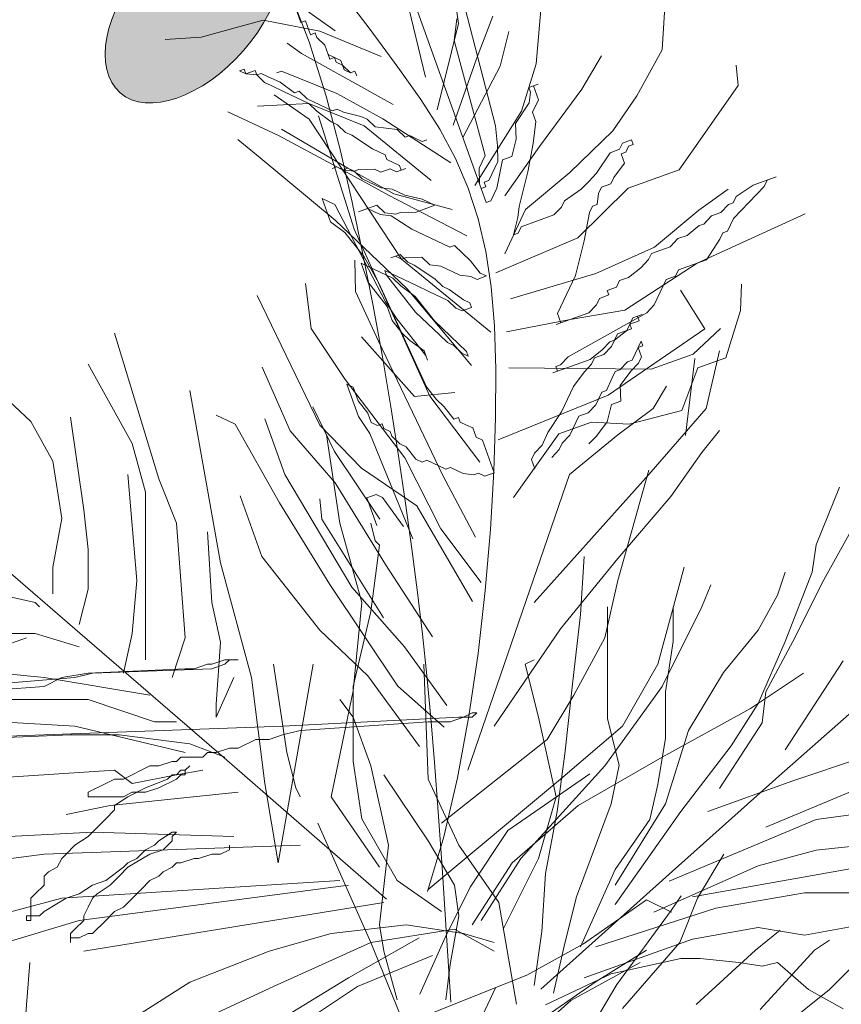
# Model space of a CAD drawing. Units: millimetres. Extents: x 595116 to 630915, y 909473 to 920225.
# Tile 101 of 134: x 629803.095 to 629807.854, y 919172.019 to 919177.721. Entities that reach past the tile are written whole.
import ezdxf

# ---------------------------------------------------------------- set-up
doc = ezdxf.new("R2010")
doc.units = ezdxf.units.MM
doc.layers.add('L-PLNT', color=85, linetype='Continuous', lineweight=13)

# ---------------------------------------------------------------- blocks, each defined once
blk = doc.blocks.new('A$C4FB75ABC')
for p, q in [((2.7169, 3.7399), (2.6018, 4.2172)), ((2.8029, 3.5683), (2.5783, 4.1926)), ((2.7679, 3.8231), (2.7507, 3.9385)), ((2.7636, 3.9026), (2.8247, 3.6653)), ((2.5777, 3.8114), (2.4796, 3.8815)), ((2.5372, 3.7949), (2.5035, 3.8821)), ((2.5794, 3.8826), (2.6314, 3.8136)), ((2.8876, 3.7608), (2.897, 3.8696)), ((2.5166, 3.8462), (2.5244, 3.8247)), ((2.4664, 3.8281), (2.3706, 3.8017)), ((2.5536, 3.8109), (2.4664, 3.8281)), ((2.7613, 3.7965), (2.7653, 3.8303)), ((2.7957, 3.7683), (2.8207, 3.834)), ((3.0823, 3.7823), (3.0858, 3.8403)), ((2.5244, 3.8247), (2.5315, 3.8272)), ((2.5315, 3.8272), (2.5393, 3.8057)), ((2.6314, 3.8136), (2.6743, 3.7558)), ((2.7349, 3.6897), (2.7679, 3.8231)), ((2.3706, 3.8017), (2.3152, 3.798)), ((2.5393, 3.8057), (2.5464, 3.8083)), ((2.5464, 3.8083), (2.549, 3.8011)), ((2.549, 3.8011), (2.5614, 3.7893)), ((2.6486, 3.7721), (2.5536, 3.8109)), ((2.8322, 3.7571), (2.8454, 3.8105)), ((2.5255, 3.7764), (2.5034, 3.7928)), ((2.5638, 3.7106), (2.5372, 3.7949)), ((2.5614, 3.7893), (2.5665, 3.775)), ((2.8089, 3.6191), (2.7613, 3.7965)), ((2.6672, 3.6978), (2.5255, 3.7764)), ((2.5665, 3.775), (2.5763, 3.7704)), ((2.5691, 3.7678), (2.5665, 3.775)), ((2.5763, 3.7704), (2.5691, 3.7678)), ((2.5763, 3.7704), (2.5789, 3.7632)), ((2.586, 3.7658), (2.5763, 3.7704)), ((2.7596, 3.6662), (2.7957, 3.7683)), ((2.9584, 3.7215), (2.9885, 3.7729)), ((3.043, 3.7114), (3.0823, 3.7823)), ((2.4369, 3.7526), (2.4297, 3.7501)), ((2.4394, 3.7455), (2.4369, 3.7526)), ((2.5789, 3.7632), (2.5886, 3.7586)), ((2.5886, 3.7586), (2.586, 3.7658)), ((2.5886, 3.7586), (2.5912, 3.7515)), ((2.601, 3.7469), (2.5886, 3.7586)), ((2.6743, 3.7558), (2.7096, 3.7056)), ((2.7745, 3.6472), (2.8322, 3.7571)), ((2.8652, 3.6879), (2.8876, 3.7608)), ((3.1994, 3.7272), (3.1962, 3.7584)), ((2.4297, 3.7501), (2.4394, 3.7455)), ((2.4538, 3.7506), (2.4394, 3.7455)), ((2.4394, 3.7455), (2.4564, 3.7435)), ((2.4564, 3.7435), (2.4538, 3.7506)), ((2.4635, 3.746), (2.4564, 3.7435)), ((2.4564, 3.7435), (2.4687, 3.7317)), ((2.4733, 3.7414), (2.4635, 3.746)), ((2.4928, 3.7323), (2.4733, 3.7414)), ((2.4948, 3.7492), (2.4876, 3.7466)), ((2.58, 3.715), (2.4948, 3.7492)), ((2.5912, 3.7515), (2.601, 3.7469)), ((2.601, 3.7469), (2.6081, 3.7494)), ((2.6081, 3.7494), (2.601, 3.7469)), ((2.6081, 3.7494), (2.6107, 3.7423)), ((2.6107, 3.7423), (2.6081, 3.7494)), ((2.4687, 3.7317), (2.4785, 3.7271)), ((2.4785, 3.7271), (2.498, 3.7179)), ((2.5149, 3.7159), (2.4928, 3.7323)), ((2.8907, 3.7295), (2.8764, 3.7244)), ((2.8764, 3.7244), (2.8789, 3.7172)), ((2.8835, 3.727), (2.8907, 3.7295)), ((2.8913, 3.7054), (2.8835, 3.727)), ((3.1085, 3.5972), (3.1994, 3.7272)), ((2.5376, 3.6754), (2.4836, 3.7127)), ((2.498, 3.7179), (2.5272, 3.7041)), ((2.5221, 3.7185), (2.5149, 3.7159)), ((2.5344, 3.7067), (2.5221, 3.7185)), ((2.5441, 3.7021), (2.5344, 3.7067)), ((2.5853, 3.6284), (2.5638, 3.7106)), ((2.6509, 3.6757), (2.58, 3.715)), ((2.8789, 3.7172), (2.8769, 3.7003)), ((2.893, 3.6331), (2.9584, 3.7215)), ((3.0058, 3.6575), (3.043, 3.7114)), ((2.537, 3.6995), (2.4575, 3.6952)), ((2.5272, 3.7041), (2.537, 3.6995)), ((2.537, 3.6995), (2.5493, 3.6877)), ((2.6222, 3.6653), (2.537, 3.6995)), ((2.5637, 3.6929), (2.5441, 3.7021)), ((2.5734, 3.6883), (2.5637, 3.6929)), ((2.7096, 3.7056), (2.7388, 3.6597)), ((2.8769, 3.7003), (2.856, 3.6684)), ((2.8821, 3.6859), (2.8913, 3.7054)), ((2.4899, 3.6502), (2.4119, 3.6869)), ((2.5493, 3.6877), (2.5714, 3.6714)), ((2.6067, 3.5058), (2.5519, 3.6806)), ((2.5806, 3.6909), (2.5734, 3.6883)), ((2.5903, 3.6863), (2.5806, 3.6909)), ((2.617, 3.6797), (2.5903, 3.6863)), ((2.6268, 3.6751), (2.617, 3.6797)), ((2.7932, 3.5729), (2.8652, 3.6879)), ((2.8873, 3.6716), (2.8821, 3.6859)), ((2.6801, 3.4593), (2.5376, 3.6754)), ((2.5714, 3.6714), (2.5812, 3.6668)), ((2.5812, 3.6668), (2.5935, 3.655)), ((2.7255, 3.5809), (2.6222, 3.6653)), ((2.6391, 3.6633), (2.6268, 3.6751)), ((2.673, 3.6593), (2.6391, 3.6633)), ((2.7562, 3.6082), (2.6509, 3.6757)), ((2.8247, 3.6653), (2.8279, 3.634)), ((2.856, 3.6684), (2.8566, 3.6443)), ((2.8833, 3.6377), (2.8873, 3.6716)), ((2.5803, 3.6016), (2.4899, 3.6502)), ((2.5972, 3.5996), (2.4945, 3.6599)), ((2.5935, 3.655), (2.6032, 3.6504)), ((2.6032, 3.6504), (2.6351, 3.6295)), ((2.6853, 3.6475), (2.673, 3.6593)), ((2.6925, 3.6501), (2.6853, 3.6475)), ((2.7022, 3.6455), (2.6925, 3.6501)), ((2.7388, 3.6597), (2.763, 3.6147)), ((2.9398, 3.5932), (3.0058, 3.6575)), ((2.4618, 3.6157), (2.4274, 3.6439)), ((2.712, 3.6409), (2.7022, 3.6455)), ((2.7192, 3.6435), (2.712, 3.6409)), ((2.8279, 3.634), (2.8285, 3.6099)), ((2.8394, 3.5571), (2.893, 3.6331)), ((2.8566, 3.6443), (2.85, 3.6176)), ((2.8746, 3.5941), (2.8833, 3.6377)), ((3.0207, 3.6385), (3.0161, 3.6288)), ((3.035, 3.6437), (3.0207, 3.6385)), ((3.0258, 3.6242), (3.0304, 3.6339)), ((3.0304, 3.6339), (3.0376, 3.6365)), ((3.0376, 3.6365), (3.035, 3.6437)), ((2.5774, 3.5196), (2.4618, 3.6157)), ((2.6037, 3.5475), (2.5853, 3.6284)), ((2.6351, 3.6295), (2.6448, 3.6249)), ((2.6448, 3.6249), (2.6546, 3.6203)), ((2.6546, 3.6203), (2.6572, 3.6131)), ((2.7998, 3.5996), (2.8089, 3.6191)), ((2.85, 3.6176), (2.8356, 3.6125)), ((3.0017, 3.6236), (2.9808, 3.5918)), ((3.0161, 3.6288), (3.0017, 3.6236)), ((3.0187, 3.6216), (3.0258, 3.6242)), ((3.0238, 3.6072), (3.0187, 3.6216)), ((2.5803, 3.6016), (2.5731, 3.5991)), ((2.5731, 3.5991), (2.5803, 3.6016)), ((2.5901, 3.597), (2.5803, 3.6016)), ((2.5803, 3.6016), (2.5901, 3.597)), ((2.6609, 3.5577), (2.5803, 3.6016)), ((2.6572, 3.6131), (2.6669, 3.6085)), ((2.6669, 3.6085), (2.6767, 3.6039)), ((2.6767, 3.6039), (2.6793, 3.5967)), ((2.763, 3.6147), (2.7827, 3.5691)), ((2.8285, 3.6099), (2.8193, 3.5904)), ((2.8356, 3.6125), (2.827, 3.5688)), ((3.0075, 3.5852), (3.0238, 3.6072)), ((2.5972, 3.5996), (2.5901, 3.597)), ((2.5901, 3.597), (2.607, 3.595)), ((2.607, 3.595), (2.5972, 3.5996)), ((2.6681, 3.5603), (2.5972, 3.5996)), ((2.6142, 3.5976), (2.607, 3.595)), ((2.607, 3.595), (2.6193, 3.5833)), ((2.6383, 3.5982), (2.6142, 3.5976)), ((2.648, 3.5936), (2.6383, 3.5982)), ((2.6623, 3.5987), (2.648, 3.5936)), ((2.6721, 3.5942), (2.6623, 3.5987)), ((2.6864, 3.5993), (2.6721, 3.5942)), ((2.6793, 3.5967), (2.6864, 3.5993)), ((2.8003, 3.5755), (2.7998, 3.5996)), ((2.8193, 3.5904), (2.8147, 3.5806)), ((2.868, 3.5674), (2.8746, 3.5941)), ((2.8712, 3.5361), (2.9398, 3.5932)), ((2.9808, 3.5918), (2.969, 3.5794)), ((3.0029, 3.5754), (3.0075, 3.5852)), ((3.0296, 3.5688), (3.1085, 3.5972)), ((3.2582, 3.5862), (3.2224, 3.5733)), ((3.2439, 3.5811), (3.2582, 3.5862)), ((2.6193, 3.5833), (2.6486, 3.5695)), ((2.8107, 3.5468), (2.8003, 3.5755)), ((2.8101, 3.5709), (2.8029, 3.5683)), ((2.8147, 3.5806), (2.8075, 3.578)), ((2.8075, 3.578), (2.8101, 3.5709)), ((2.969, 3.5794), (2.9573, 3.5671)), ((2.984, 3.5605), (2.9885, 3.5702)), ((2.9885, 3.5702), (3.0029, 3.5754)), ((3.2224, 3.5733), (3.1962, 3.5558)), ((3.2158, 3.5466), (3.2393, 3.5713)), ((3.2393, 3.5713), (3.2439, 3.5811)), ((2.6486, 3.5695), (2.6655, 3.5675)), ((2.7805, 3.4954), (2.6609, 3.5577)), ((2.6655, 3.5675), (2.685, 3.5583)), ((2.7579, 3.5359), (2.6681, 3.5603)), ((2.685, 3.5583), (2.7117, 3.5517)), ((2.7827, 3.5691), (2.7983, 3.5216)), ((2.8224, 3.5591), (2.8178, 3.5493)), ((2.827, 3.5688), (2.8224, 3.5591)), ((2.8614, 3.5407), (2.868, 3.5674)), ((2.9573, 3.5671), (2.9312, 3.5496)), ((2.9518, 3.4922), (3.0296, 3.5688)), ((2.9819, 3.5435), (2.984, 3.5605)), ((3.1389, 3.5352), (3.1839, 3.5676)), ((3.1962, 3.5558), (3.1917, 3.5461)), ((2.5671, 3.5483), (2.5573, 3.5529)), ((2.5573, 3.5529), (2.5703, 3.517)), ((2.5769, 3.5437), (2.5671, 3.5483)), ((2.6552, 3.3935), (2.5769, 3.5437)), ((2.6204, 3.467), (2.6037, 3.5475)), ((2.642, 3.5428), (2.6133, 3.5325)), ((2.6543, 3.531), (2.642, 3.5428)), ((2.7312, 3.5425), (2.7025, 3.5321)), ((2.7117, 3.5517), (2.7214, 3.5471)), ((2.7214, 3.5471), (2.7312, 3.5425)), ((2.8178, 3.5493), (2.8107, 3.5468)), ((2.8594, 3.5238), (2.8614, 3.5407)), ((2.9266, 3.5398), (2.9148, 3.5275)), ((2.9312, 3.5496), (2.9266, 3.5398)), ((2.9702, 3.5312), (2.9748, 3.541)), ((2.9748, 3.541), (2.9819, 3.5435)), ((3.1845, 3.5435), (3.1727, 3.5311)), ((3.1917, 3.5461), (3.1845, 3.5435)), ((3.1922, 3.522), (3.2158, 3.5466)), ((2.6133, 3.5325), (2.6276, 3.5376)), ((2.6276, 3.5376), (2.6471, 3.5284)), ((2.6471, 3.5284), (2.6641, 3.5264)), ((2.6712, 3.529), (2.6543, 3.531)), ((2.6641, 3.5264), (2.6959, 3.5055)), ((2.6784, 3.5316), (2.6712, 3.529)), ((2.7025, 3.5321), (2.6784, 3.5316)), ((2.8391, 3.4678), (2.8712, 3.5361)), ((2.9148, 3.5275), (2.8646, 3.5094)), ((2.9616, 3.4876), (2.9702, 3.5312)), ((3.0703, 3.4781), (3.1389, 3.5352)), ((3.136, 3.4531), (3.303, 3.5294)), ((3.1584, 3.526), (3.1466, 3.5136)), ((3.1727, 3.5311), (3.1584, 3.526)), ((2.5703, 3.517), (2.5924, 3.5006)), ((2.6885, 3.4136), (2.5774, 3.5196)), ((2.7983, 3.5216), (2.81, 3.4712)), ((2.8528, 3.4971), (2.8594, 3.5238)), ((2.8646, 3.5094), (2.86, 3.4997)), ((3.1394, 3.5111), (3.1205, 3.4961)), ((3.1466, 3.5136), (3.1394, 3.5111)), ((3.1831, 3.5024), (3.1922, 3.522)), ((2.5924, 3.5006), (2.6222, 3.4627)), ((2.7237, 3.248), (2.6067, 3.5058)), ((2.6959, 3.5055), (2.7154, 3.4963)), ((2.7154, 3.4963), (2.7252, 3.4917)), ((2.86, 3.4997), (2.8528, 3.4971)), ((3.1205, 3.4961), (3.1062, 3.491)), ((3.1713, 3.4901), (3.1759, 3.4999)), ((3.1759, 3.4999), (3.1831, 3.5024)), ((2.7252, 3.4917), (2.7544, 3.4779)), ((2.7544, 3.4779), (2.7616, 3.4805)), ((2.7616, 3.4805), (2.774, 3.4687)), ((2.8253, 3.4385), (2.9518, 3.4922)), ((2.9484, 3.4342), (2.9616, 3.4876)), ((3.0944, 3.4786), (3.0657, 3.4683)), ((3.1062, 3.491), (3.0944, 3.4786)), ((3.1503, 3.4583), (3.1713, 3.4901)), ((2.636, 3.3873), (2.6204, 3.467)), ((2.6632, 3.4613), (2.6776, 3.4664)), ((2.6704, 3.4639), (2.6632, 3.4613)), ((2.6801, 3.4593), (2.6704, 3.4639)), ((2.6776, 3.4664), (2.6899, 3.4547)), ((2.774, 3.4687), (2.7863, 3.4569)), ((2.81, 3.4712), (2.8183, 3.4166)), ((2.9797, 3.4374), (3.0703, 3.4781)), ((3.0657, 3.4683), (3.0611, 3.4586)), ((2.609, 3.4093), (2.6078, 3.4576)), ((2.6566, 3.4346), (2.6176, 3.453)), ((2.6176, 3.453), (2.6279, 3.4243)), ((2.6222, 3.4627), (2.6449, 3.4222)), ((2.6873, 3.4618), (2.6801, 3.4593)), ((2.8178, 3.3467), (2.6801, 3.4593)), ((2.7114, 3.4624), (2.6873, 3.4618)), ((2.6899, 3.4547), (2.6996, 3.4501)), ((2.6996, 3.4501), (2.7315, 3.4291)), ((2.7237, 3.4506), (2.7114, 3.4624)), ((2.7407, 3.4486), (2.7237, 3.4506)), ((2.7699, 3.4348), (2.7407, 3.4486)), ((2.7863, 3.4569), (2.8012, 3.438)), ((3.0244, 3.3805), (3.136, 3.4531)), ((3.0611, 3.4586), (3.0494, 3.4462)), ((3.1073, 3.4428), (3.1503, 3.4583)), ((2.6638, 3.4372), (2.654, 3.4418)), ((2.654, 3.4418), (2.6566, 3.4346)), ((2.6566, 3.4346), (2.6664, 3.43)), ((2.6865, 3.3967), (2.6566, 3.4346)), ((2.693, 3.4234), (2.6638, 3.4372)), ((2.7869, 3.4328), (2.7699, 3.4348)), ((2.811, 3.4334), (2.7966, 3.4282)), ((2.8012, 3.438), (2.811, 3.4334)), ((2.848, 3.3981), (2.9797, 3.4374)), ((2.9392, 3.4147), (2.9484, 3.4342)), ((3.0494, 3.4462), (3.0304, 3.4313)), ((3.1027, 3.433), (3.1073, 3.4428)), ((2.5404, 3.3522), (2.5315, 3.422)), ((2.6279, 3.4243), (2.6578, 3.3864)), ((2.6449, 3.4222), (2.7186, 3.2624)), ((2.6664, 3.43), (2.6787, 3.4182)), ((2.6787, 3.4182), (2.7008, 3.4019)), ((2.7028, 3.4188), (2.693, 3.4234)), ((2.7223, 3.4096), (2.7028, 3.4188)), ((2.7315, 3.4291), (2.7438, 3.4173)), ((2.7966, 3.4282), (2.7869, 3.4328)), ((3.0161, 3.4262), (3.0115, 3.4164)), ((3.0304, 3.4313), (3.0161, 3.4262)), ((3.07, 3.3888), (3.0884, 3.4279)), ((3.0884, 3.4279), (3.1027, 3.433)), ((3.2028, 3.3799), (3.2043, 3.4209)), ((2.5536, 3.203), (2.4572, 3.4034)), ((2.6446, 3.333), (2.609, 3.4093)), ((2.7877, 3.2953), (2.6885, 3.4136)), ((2.7516, 3.3958), (2.7223, 3.4096)), ((2.7438, 3.4173), (2.7536, 3.4127)), ((2.7536, 3.4127), (2.7757, 3.3964)), ((2.8183, 3.4166), (2.8233, 3.3565)), ((2.9254, 3.3854), (2.9392, 3.4147)), ((2.9997, 3.4041), (2.9854, 3.3989)), ((3.0115, 3.4164), (2.9972, 3.4112)), ((2.9972, 3.4112), (2.9997, 3.4041)), ((3.1481, 3.3521), (3.1105, 3.4115)), ((2.6727, 3.3674), (2.6552, 3.3935)), ((2.7014, 3.3777), (2.6865, 3.3967)), ((2.7008, 3.4019), (2.7306, 3.364)), ((2.7639, 3.384), (2.7516, 3.3958)), ((2.7757, 3.3964), (2.7854, 3.3918)), ((2.7854, 3.3918), (2.788, 3.3846)), ((2.9808, 3.3891), (2.969, 3.3768)), ((2.9854, 3.3989), (2.9808, 3.3891)), ((3.0583, 3.3765), (3.07, 3.3888)), ((2.6503, 3.3086), (2.636, 3.3873)), ((2.6578, 3.3864), (2.6655, 3.3648)), ((2.7384, 3.3424), (2.7014, 3.3777)), ((2.7737, 3.3794), (2.7639, 3.384)), ((2.788, 3.3846), (2.7737, 3.3794)), ((2.969, 3.3768), (2.9188, 3.3587)), ((2.9208, 3.3757), (2.9254, 3.3854)), ((2.926, 3.3613), (2.9208, 3.3757)), ((2.9369, 3.3085), (3.0583, 3.3765)), ((2.9403, 3.3665), (3.0244, 3.3805)), ((3.0511, 3.3739), (3.0367, 3.3687)), ((3.0439, 3.3713), (3.0511, 3.3739)), ((3.1805, 3.307), (3.2028, 3.3799)), ((2.6655, 3.3648), (2.6804, 3.3459)), ((2.7174, 3.3106), (2.6727, 3.3674)), ((2.7306, 3.364), (2.743, 3.3522)), ((2.8419, 3.3473), (2.9403, 3.3665)), ((2.9188, 3.3587), (2.926, 3.3613)), ((3.0322, 3.359), (3.0276, 3.3492)), ((3.0367, 3.3687), (3.0322, 3.359)), ((3.0322, 3.359), (3.0465, 3.3642)), ((3.0347, 3.3518), (3.0322, 3.359)), ((3.0465, 3.3642), (3.0439, 3.3713)), ((2.2372, 3.345), (2.3054, 3.1203)), ((2.5929, 3.2739), (2.5404, 3.3522)), ((2.6804, 3.3459), (2.6928, 3.3341)), ((2.7507, 3.3307), (2.7384, 3.3424)), ((2.743, 3.3522), (2.7553, 3.3404)), ((2.8233, 3.3565), (2.8254, 3.2898)), ((2.9986, 3.2497), (3.1481, 3.3521)), ((3.0276, 3.3492), (3.0086, 3.3343)), ((3.0086, 3.3343), (3.0132, 3.3441)), ((3.0132, 3.3441), (3.0347, 3.3518)), ((3.1297, 3.313), (3.1722, 3.3526)), ((2.6997, 3.2474), (2.6179, 3.3396)), ((2.7435, 3.1255), (2.6446, 3.333)), ((2.6928, 3.3341), (2.7149, 3.3178)), ((2.7605, 3.3261), (2.7507, 3.3307)), ((2.7553, 3.3404), (2.78, 3.3169)), ((3.0015, 3.3317), (2.9897, 3.3194)), ((3.0086, 3.3343), (3.0015, 3.3317)), ((3.004, 3.3246), (3.0086, 3.3343)), ((3.0497, 3.3329), (3.0451, 3.3231)), ((3.0522, 3.3257), (3.0497, 3.3329)), ((2.7149, 3.3178), (2.72, 3.3034)), ((2.7728, 3.3143), (2.7605, 3.3261)), ((2.7826, 3.3097), (2.7728, 3.3143)), ((2.78, 3.3169), (2.7826, 3.3097)), ((2.9897, 3.3194), (2.9708, 3.3045)), ((2.9779, 3.3071), (2.9923, 3.3122)), ((2.9923, 3.3122), (3.004, 3.3246)), ((3.0359, 3.3036), (3.0405, 3.3134)), ((3.0405, 3.3134), (3.0451, 3.3231)), ((3.0451, 3.3231), (3.0522, 3.3257)), ((3.0451, 3.3231), (3.0502, 3.3088)), ((3.0651, 3.2898), (3.1297, 3.313)), ((3.1501, 3.2292), (3.1706, 3.3178)), ((1.9988, 3.3109), (2.1078, 3.2088)), ((2.1963, 3.2973), (2.2645, 3.1748)), ((2.6635, 3.2315), (2.6503, 3.3086)), ((2.72, 3.3034), (2.7174, 3.3106)), ((2.9708, 3.3045), (2.9134, 3.2838)), ((2.9251, 3.2962), (2.9369, 3.3085)), ((2.9616, 3.285), (2.9733, 3.2973)), ((2.9733, 3.2973), (2.9779, 3.3071)), ((3.0169, 3.2887), (3.0287, 3.301)), ((3.0287, 3.301), (3.0359, 3.3036)), ((3.0456, 3.299), (3.0339, 3.2867)), ((3.0502, 3.3088), (3.0456, 3.299)), ((3.1303, 3.2889), (3.1323, 3.3059)), ((3.1374, 3.2915), (3.1805, 3.307)), ((2.508, 3.1947), (2.4647, 3.2926)), ((2.8254, 3.2898), (2.825, 3.2153)), ((2.8457, 3.2919), (3.0651, 3.2898)), ((2.9134, 3.2838), (2.9206, 3.2864)), ((2.918, 3.2936), (2.9251, 3.2962)), ((2.9206, 3.2864), (2.918, 3.2936)), ((2.9452, 3.2629), (2.9616, 3.285)), ((3.0052, 3.2763), (3.0098, 3.2861)), ((3.0098, 3.2861), (3.0169, 3.2887)), ((3.0339, 3.2867), (3.0175, 3.2646)), ((3.1125, 3.2258), (3.1374, 3.2915)), ((3.1182, 3.1873), (3.1303, 3.2889)), ((2.685, 3.153), (2.5929, 3.2739)), ((2.6053, 3.2621), (2.5955, 3.2667)), ((2.5955, 3.2667), (2.6136, 3.2165)), ((2.996, 3.2568), (3.0052, 3.2763)), ((2.353, 3.2565), (2.4007, 2.9909)), ((2.613, 3.2406), (2.6053, 3.2621)), ((2.7622, 3.2537), (2.6997, 3.2474)), ((2.7186, 3.2624), (2.7335, 3.2434)), ((2.936, 3.2434), (2.9452, 3.2629)), ((2.9842, 3.2445), (2.9888, 3.2542)), ((2.9888, 3.2542), (2.996, 3.2568)), ((3.0175, 3.2646), (3.0181, 3.2405)), ((3.0684, 3.2292), (3.0888, 3.2633)), ((2.6279, 3.2216), (2.613, 3.2406)), ((2.8009, 3.1461), (2.7237, 3.248)), ((2.7335, 3.2434), (2.7458, 3.2316)), ((2.829, 3.1805), (2.9986, 3.2497)), ((2.9269, 3.2238), (2.936, 3.2434)), ((2.9797, 3.2347), (2.9842, 3.2445)), ((3.0181, 3.2405), (3.0038, 3.2353)), ((2.5763, 3.1625), (2.5433, 3.2317)), ((2.6331, 3.2073), (2.6279, 3.2216)), ((2.6754, 3.1561), (2.6635, 3.2315)), ((2.7458, 3.2316), (2.7608, 3.2127)), ((2.9059, 3.192), (2.9269, 3.2238)), ((2.9535, 3.2172), (2.9679, 3.2224)), ((2.9679, 3.2224), (2.9797, 3.2347)), ((3.0038, 3.2353), (2.9972, 3.2086)), ((3.0139, 3.1884), (3.0684, 3.2292)), ((3.031, 3.2046), (3.1125, 3.2258)), ((3.0616, 3.1271), (3.1501, 3.2292)), ((2.1078, 3.2088), (2.1418, 3.1475)), ((2.1691, 3.2156), (2.1895, 3.0726)), ((2.4234, 3.2048), (2.3941, 3.2186)), ((2.5, 3.127), (2.469, 3.2131)), ((2.6136, 3.2165), (2.6311, 3.1904)), ((2.6428, 3.2027), (2.6331, 3.2073)), ((2.65, 3.2053), (2.6428, 3.2027)), ((2.6526, 3.1981), (2.65, 3.2053)), ((2.7608, 3.2127), (2.7679, 3.2153)), ((2.7679, 3.2153), (2.7705, 3.2081)), ((2.7705, 3.2081), (2.7803, 3.2035)), ((2.825, 3.2153), (2.8223, 3.1323)), ((2.9229, 3.19), (2.9731, 3.208)), ((2.9398, 3.188), (2.949, 3.2075)), ((2.949, 3.2075), (2.9535, 3.2172)), ((2.9731, 3.208), (3.031, 3.2046)), ((2.9972, 3.2086), (2.9808, 3.1865)), ((2.4914, 3.0833), (2.4234, 3.2048)), ((2.5774, 3.1143), (2.508, 3.1947)), ((2.6179, 3.137), (2.5536, 3.203)), ((2.6311, 3.1904), (2.6976, 3.0279)), ((2.6624, 3.1935), (2.6526, 3.1981)), ((2.6649, 3.1863), (2.6624, 3.1935)), ((2.7803, 3.2035), (2.79, 3.1989)), ((2.79, 3.1989), (2.7952, 3.1846)), ((2.8967, 3.1725), (2.9059, 3.192)), ((3.1433, 3.1611), (3.1706, 3.1952)), ((2.5847, 3.0522), (2.5642, 3.1884)), ((2.6773, 3.1746), (2.6649, 3.1863)), ((2.7952, 3.1846), (2.8049, 3.18)), ((2.8049, 3.18), (2.823, 3.1297)), ((2.8529, 3.0918), (2.9229, 3.19)), ((2.9234, 3.1659), (2.928, 3.1756)), ((2.928, 3.1756), (2.9398, 3.188)), ((2.9389, 3.1271), (3.0139, 3.1884)), ((2.9808, 3.1865), (2.969, 3.1742)), ((2.2645, 3.1748), (2.2849, 3.0999)), ((2.6463, 3.058), (2.5763, 3.1625)), ((2.687, 3.17), (2.6773, 3.1746)), ((2.7019, 3.151), (2.687, 3.17)), ((2.8804, 3.1504), (2.885, 3.1601)), ((2.885, 3.1601), (2.8967, 3.1725)), ((2.9117, 3.1535), (2.9234, 3.1659)), ((3.0956, 3.093), (3.1433, 3.1611)), ((2.1418, 3.1475), (2.1555, 3.059)), ((2.6863, 3.0831), (2.6754, 3.1561)), ((2.7407, 3.0434), (2.685, 3.153)), ((2.7117, 3.1464), (2.7019, 3.151)), ((2.7189, 3.149), (2.7117, 3.1464)), ((2.7286, 3.1444), (2.7189, 3.149)), ((2.8856, 3.136), (2.8804, 3.1504)), ((2.7037, 3.0787), (2.6179, 3.137)), ((2.7481, 3.1352), (2.7286, 3.1444)), ((2.7553, 3.1378), (2.7481, 3.1352)), ((2.7651, 3.1332), (2.7553, 3.1378)), ((2.7748, 3.1286), (2.7651, 3.1332)), ((2.823, 3.1297), (2.8087, 3.1246)), ((2.8223, 3.1323), (2.817, 3.0425)), ((3.0139, 2.9637), (3.0616, 3.1339)), ((2.2577, 3.1271), (2.2713, 2.9637)), ((2.3054, 3.1203), (2.3326, 3.0522)), ((2.603, 2.9533), (2.5, 3.127)), ((2.6552, 2.9883), (2.5774, 3.1143)), ((2.794, 3.0302), (2.7435, 3.1255)), ((2.7917, 3.1266), (2.7748, 3.1286)), ((2.7823, 2.6709), (2.9389, 3.1271)), ((2.7989, 3.1292), (2.7917, 3.1266)), ((2.8087, 3.1246), (2.7989, 3.1292)), ((2.8844, 2.9296), (3.0616, 3.1271)), ((2.2849, 3.0999), (2.2849, 2.9024)), ((3.3198, 3.0184), (3.3556, 3.1078)), ((2.4644, 3.0007), (2.4308, 3.094)), ((2.5571, 3.0584), (2.5539, 3.0896)), ((2.6406, 3.0965), (2.6262, 3.0913)), ((2.6262, 3.0913), (2.6417, 3.0483)), ((2.6503, 3.0919), (2.6406, 3.0965)), ((2.6827, 3.0468), (2.6503, 3.0919)), ((3.0139, 2.9977), (3.0956, 3.093)), ((2.1895, 3.0726), (2.1963, 3.0113)), ((2.5691, 2.9573), (2.4914, 3.0833)), ((2.696, 3.0126), (2.6863, 3.0831)), ((2.7892, 2.9311), (2.7037, 3.0787)), ((3.3317, 2.9647), (3.3914, 3.072)), ((2.1555, 3.059), (2.1418, 2.9841)), ((2.6523, 2.9062), (2.5571, 3.0584)), ((2.3326, 3.0522), (2.3462, 2.8751)), ((2.3803, 3.0386), (2.3871, 2.9296)), ((2.6187, 2.9296), (2.5847, 3.0522)), ((2.6392, 3.0249), (2.6324, 3.0522)), ((2.8029, 2.9604), (2.7407, 3.0434)), ((2.817, 3.0425), (2.809, 2.948)), ((2.1835, 2.8826), (2.0174, 3.0255)), ((2.646, 3.0181), (2.6392, 3.0249)), ((2.1963, 3.0113), (2.1963, 2.95)), ((2.6324, 2.916), (2.646, 3.0181)), ((2.7046, 2.9452), (2.696, 3.0126)), ((3.3138, 2.9766), (3.3198, 3.0184)), ((2.5539, 2.887), (2.4644, 3.0007)), ((2.9253, 2.8888), (3.0139, 2.9977)), ((2.9559, 2.911), (2.9619, 3.0005)), ((2.1418, 2.9841), (2.1418, 2.9432)), ((2.4007, 2.9909), (2.4484, 2.8139)), ((2.7278, 2.8766), (2.6552, 2.9883)), ((3.0752, 2.8343), (3.1161, 2.9841)), ((2.2713, 2.9637), (2.2645, 2.882)), ((2.9935, 2.8751), (3.0139, 2.9637)), ((3.2601, 2.9408), (3.2721, 2.9766)), ((3.2721, 2.8693), (3.3138, 2.9766)), ((3.284, 2.8693), (3.3317, 2.9647)), ((2.1963, 2.95), (2.1827, 2.8956)), ((2.6741, 2.8006), (2.5691, 2.9573)), ((2.6847, 2.8611), (2.603, 2.9533)), ((2.809, 2.948), (2.7981, 2.8512)), ((3.1433, 2.9228), (3.157, 2.9569)), ((2.0533, 2.9432), (2.1146, 2.9296)), ((2.7122, 2.8807), (2.7046, 2.9452)), ((3.2303, 2.8872), (3.2601, 2.9408)), ((2.1146, 2.9296), (2.1214, 2.9228)), ((2.3871, 2.9296), (2.4007, 2.8683)), ((2.6051, 2.7934), (2.6187, 2.9296)), ((2.9977, 2.8216), (2.9977, 2.923)), ((3.082, 2.8002), (3.1433, 2.9228)), ((3.0991, 2.8693), (3.0991, 2.923)), ((2.2849, 2.9024), (2.2849, 2.8411)), ((2.6051, 2.8002), (2.6324, 2.916)), ((2.944, 2.8037), (2.9559, 2.911)), ((2.6279, 2.8164), (2.5539, 2.887)), ((2.8231, 2.739), (2.9253, 2.8888)), ((3.1766, 2.8216), (3.2303, 2.8872)), ((1.917, 2.882), (2.1146, 2.882)), ((2.101, 2.8751), (2.0056, 2.8411)), ((2.1146, 2.882), (2.1827, 2.8615)), ((2.3943, 2.7002), (2.1835, 2.8826)), ((2.2645, 2.882), (2.2508, 2.8207)), ((2.3462, 2.8751), (2.3258, 2.8139)), ((2.7189, 2.8171), (2.7122, 2.8807)), ((2.9458, 2.7866), (2.9935, 2.8751)), ((2.4007, 2.8683), (2.3939, 2.773)), ((2.7496, 2.771), (2.6847, 2.8611)), ((3.0872, 2.7918), (3.0991, 2.8693)), ((3.2303, 2.7739), (3.2721, 2.8693)), ((3.2422, 2.7918), (3.284, 2.8693)), ((2.3871, 2.8343), (2.4075, 2.8411)), ((2.4075, 2.8411), (2.428, 2.8411)), ((2.4144, 2.8411), (2.4075, 2.8343)), ((2.428, 2.8411), (2.4144, 2.8411)), ((2.7981, 2.8512), (2.784, 2.7542)), ((2.8708, 2.8343), (2.8844, 2.8411)), ((2.1963, 2.8207), (2.3462, 2.8275)), ((2.3871, 2.8275), (2.2032, 2.8207)), ((2.3462, 2.8275), (2.3599, 2.8275)), ((2.3599, 2.8275), (2.3803, 2.8343)), ((2.3803, 2.8343), (2.3871, 2.8343)), ((2.4075, 2.8343), (2.3871, 2.8275)), ((2.4825, 2.8343), (2.5029, 2.6981)), ((2.4893, 2.5279), (2.5438, 2.8343)), ((2.7209, 2.6572), (2.7141, 2.8343)), ((2.8913, 2.7526), (2.8708, 2.8343)), ((3.0207, 2.739), (3.0752, 2.8343)), ((3.2721, 2.7024), (3.3615, 2.8395)), ((2.1759, 2.8139), (2.0056, 2.8002)), ((2.0601, 2.8207), (2.1282, 2.8139)), ((2.1282, 2.8002), (2.1555, 2.8139)), ((2.1282, 2.8139), (2.2917, 2.7866)), ((2.1555, 2.8139), (2.1963, 2.8207)), ((2.2032, 2.8207), (2.1759, 2.8139)), ((2.3939, 2.7526), (2.4212, 2.8139)), ((2.4484, 2.8139), (2.4689, 2.6504)), ((2.7077, 2.7073), (2.6279, 2.8164)), ((2.7251, 2.7519), (2.7189, 2.8171)), ((2.9977, 2.7501), (2.9977, 2.8216)), ((3.1229, 2.7322), (3.1766, 2.8216)), ((3.2183, 2.7662), (3.3, 2.8207)), ((1.9443, 2.7866), (2.1282, 2.8002)), ((2.6051, 2.6845), (2.6051, 2.8002)), ((2.7456, 2.7371), (2.6741, 2.8006)), ((2.9321, 2.6964), (2.944, 2.8037)), ((2.9935, 2.6777), (3.082, 2.8002)), ((2.5711, 2.63), (2.6051, 2.7934)), ((2.9049, 2.7185), (2.9458, 2.7866)), ((3.0872, 2.7203), (3.0872, 2.7918)), ((3.2363, 2.7441), (3.2422, 2.7918)), ((2.0601, 2.7798), (2.1078, 2.7798)), ((2.1078, 2.7798), (2.1963, 2.7798)), ((2.1963, 2.7798), (2.2985, 2.7458)), ((2.3939, 2.773), (2.3939, 2.7526)), ((2.6051, 2.7526), (2.5847, 2.7798)), ((3.082, 2.6913), (3.2183, 2.7662)), ((3.1886, 2.7083), (3.2303, 2.7739)), ((3.2623, 2.6619), (3.3951, 2.779)), ((2.4961, 2.739), (2.7686, 2.7526)), ((2.6324, 2.6777), (2.6051, 2.7526)), ((2.7309, 2.6826), (2.7251, 2.7519)), ((2.7754, 2.7526), (2.755, 2.7458)), ((2.784, 2.7542), (2.7664, 2.6591)), ((2.7686, 2.7526), (2.7891, 2.7526)), ((2.7891, 2.7594), (2.7754, 2.7526)), ((2.7891, 2.7526), (2.7959, 2.7594)), ((2.7959, 2.7594), (2.7891, 2.7594)), ((2.9185, 2.63), (2.8913, 2.7526)), ((3.0156, 2.6785), (2.9977, 2.7501)), ((2.1759, 2.739), (2.0601, 2.7458)), ((2.3462, 2.6981), (2.1759, 2.739)), ((2.2985, 2.7458), (2.3326, 2.7458)), ((2.3122, 2.7321), (2.4961, 2.739)), ((2.7209, 2.7458), (2.5234, 2.7321)), ((2.755, 2.7458), (2.7209, 2.7458)), ((2.9253, 2.6572), (3.0207, 2.739)), ((3.1707, 2.6428), (3.2363, 2.7441)), ((1.8285, 2.7117), (2.1691, 2.7253)), ((1.9443, 2.7185), (2.1282, 2.7253)), ((2.1282, 2.7253), (2.3122, 2.7321)), ((2.1691, 2.7253), (2.244, 2.7253)), ((2.244, 2.7253), (2.353, 2.7117)), ((2.4961, 2.7253), (2.4757, 2.7185)), ((2.5234, 2.7321), (2.4961, 2.7253)), ((3.0752, 2.6487), (3.0872, 2.7203)), ((3.0872, 2.6189), (3.1229, 2.7322)), ((2.353, 2.7117), (2.4075, 2.6913)), ((2.4144, 2.7049), (2.3939, 2.6981)), ((2.428, 2.7049), (2.4144, 2.7049)), ((2.4552, 2.7185), (2.428, 2.7049)), ((2.4757, 2.7185), (2.4552, 2.7185)), ((2.7414, 2.5891), (2.9049, 2.7185)), ((3.111, 2.607), (3.1886, 2.7083)), ((2.3394, 2.6913), (2.3326, 2.6845)), ((2.3735, 2.6913), (2.3394, 2.6913)), ((2.3803, 2.6981), (2.3735, 2.6913)), ((2.3939, 2.6981), (2.3803, 2.6981)), ((2.6566, 2.472), (2.3943, 2.7002)), ((2.5029, 2.6981), (2.5166, 2.6436)), ((2.9201, 2.607), (2.9321, 2.6964)), ((2.9526, 2.6164), (3.082, 2.6913)), ((3.2422, 2.5831), (3.4987, 2.6904)), ((3.284, 2.6547), (3.3914, 2.6904)), ((2.2917, 2.6777), (2.2508, 2.6572)), ((2.3054, 2.6777), (2.2917, 2.6777)), ((2.3258, 2.6845), (2.3054, 2.6777)), ((2.3326, 2.6845), (2.3258, 2.6845)), ((2.3462, 2.6709), (2.353, 2.6777)), ((2.353, 2.6777), (2.3462, 2.6709)), ((2.6187, 2.596), (2.6051, 2.6845)), ((2.6596, 2.5551), (2.6324, 2.6777)), ((2.7367, 2.6065), (2.7309, 2.6826)), ((2.864, 2.5347), (2.9935, 2.6777)), ((3.0036, 2.6189), (3.0156, 2.6785)), ((1.917, 2.6504), (2.2372, 2.6709)), ((2.2372, 2.6709), (2.2645, 2.6504)), ((2.2645, 2.6504), (2.3326, 2.664)), ((2.3258, 2.664), (2.319, 2.6572)), ((2.3326, 2.664), (2.3258, 2.664)), ((2.3394, 2.6709), (2.3326, 2.664)), ((2.3326, 2.664), (2.3735, 2.6709)), ((2.3326, 2.6572), (2.3394, 2.664)), ((2.3462, 2.6709), (2.3394, 2.6709)), ((2.3394, 2.664), (2.3462, 2.664)), ((2.3462, 2.664), (2.3462, 2.6709)), ((2.6528, 2.664), (2.7209, 2.5619)), ((2.7664, 2.6591), (2.7451, 2.5683)), ((2.8442, 2.5778), (2.9704, 2.6651)), ((3.0976, 2.5149), (3.2623, 2.6619)), ((2.2236, 2.6504), (2.1963, 2.6368)), ((2.2372, 2.6572), (2.2236, 2.6504)), ((2.2508, 2.6572), (2.2372, 2.6572)), ((2.2849, 2.6436), (2.2577, 2.63)), ((2.319, 2.6572), (2.2849, 2.6436)), ((2.2849, 2.6368), (2.3054, 2.6436)), ((2.3054, 2.6436), (2.3326, 2.6572)), ((2.4689, 2.6504), (2.4893, 2.5279)), ((2.5166, 2.6436), (2.5234, 2.63)), ((2.7209, 2.487), (2.9253, 2.6572)), ((2.7686, 2.5551), (2.7209, 2.6572)), ((3.0633, 2.5951), (3.0752, 2.6487)), ((3.1528, 2.607), (3.284, 2.6547)), ((2.1963, 2.6368), (2.1963, 2.63)), ((2.1963, 2.63), (2.2508, 2.63)), ((2.428, 2.6368), (2.2304, 2.6164)), ((2.2577, 2.63), (2.2372, 2.6164)), ((2.2508, 2.63), (2.2645, 2.6368)), ((2.2645, 2.6368), (2.2849, 2.6368)), ((2.646, 2.5211), (2.5711, 2.63)), ((2.8913, 2.5347), (2.9185, 2.63)), ((2.2304, 2.6164), (2.1623, 2.6028)), ((2.2372, 2.6164), (2.2372, 2.6096)), ((2.8504, 2.5279), (2.9526, 2.6164)), ((2.95, 2.4758), (3.0036, 2.6189)), ((3.0096, 2.4937), (3.0872, 2.6189)), ((3.3198, 2.5951), (3.457, 2.6129)), ((2.2372, 2.6096), (2.2236, 2.596)), ((2.7426, 2.5213), (2.7367, 2.6065)), ((2.9022, 2.5116), (2.9201, 2.607)), ((3.0096, 2.4639), (3.111, 2.607)), ((2.2236, 2.596), (2.21, 2.5823)), ((2.5506, 2.5891), (2.6324, 2.4053)), ((2.6732, 2.5006), (2.6187, 2.596)), ((3.0096, 2.5176), (3.0633, 2.5951)), ((3.0931, 2.4997), (3.3198, 2.5951)), ((2.2032, 2.5755), (2.0737, 2.5687)), ((2.1963, 2.5687), (2.1759, 2.5551)), ((2.21, 2.5823), (2.1963, 2.5687)), ((2.4212, 2.5687), (2.2032, 2.5755)), ((2.3054, 2.5619), (2.3258, 2.5755)), ((2.3258, 2.5755), (2.3326, 2.5755)), ((2.3326, 2.5755), (2.3258, 2.5687)), ((2.3258, 2.5687), (2.3258, 2.5619)), ((2.7451, 2.5683), (2.72, 2.484)), ((2.786, 2.4905), (2.8442, 2.5778)), ((2.5234, 2.5551), (2.1282, 2.5415)), ((2.1759, 2.5551), (2.1623, 2.5415)), ((2.2849, 2.5483), (2.2985, 2.5551)), ((2.2985, 2.5551), (2.3054, 2.5619)), ((2.3258, 2.5619), (2.3122, 2.5483)), ((2.4144, 2.5483), (2.4144, 2.5551)), ((2.646, 2.4325), (2.6596, 2.5551)), ((2.7209, 2.5619), (2.7618, 2.4938)), ((2.8299, 2.4666), (2.7686, 2.5551)), ((3.3198, 2.5474), (3.4272, 2.5593)), ((2.1282, 2.5415), (1.9715, 2.5211)), ((2.1623, 2.5415), (2.1555, 2.5347)), ((2.2917, 2.5415), (2.2577, 2.5211)), ((2.2713, 2.5347), (2.2781, 2.5415)), ((2.2781, 2.5415), (2.2849, 2.5483)), ((2.3122, 2.5483), (2.2917, 2.5415)), ((2.3667, 2.5347), (2.3871, 2.5415)), ((2.3871, 2.5415), (2.4007, 2.5415)), ((2.4007, 2.5415), (2.4144, 2.5483)), ((3.1289, 2.4758), (3.5345, 2.5474)), ((3.1365, 2.4734), (3.1774, 2.5415)), ((3.2303, 2.5235), (3.3198, 2.5474)), ((2.1555, 2.5347), (2.1487, 2.5211)), ((2.2508, 2.5211), (2.2577, 2.5279)), ((2.2577, 2.5279), (2.2713, 2.5347)), ((2.3258, 2.5211), (2.3326, 2.5279)), ((2.3326, 2.5279), (2.3394, 2.5279)), ((2.3394, 2.5279), (2.3599, 2.5347)), ((2.3599, 2.5347), (2.3667, 2.5347)), ((2.7891, 2.4325), (2.8504, 2.5279)), ((2.8027, 2.4393), (2.864, 2.5347)), ((2.8368, 2.4257), (2.8913, 2.5347)), ((3.0693, 2.452), (3.2303, 2.5235)), ((2.135, 2.5142), (2.1282, 2.5074)), ((2.1282, 2.5074), (2.1282, 2.4938)), ((2.1487, 2.5211), (2.135, 2.5142)), ((2.2236, 2.5006), (2.2508, 2.5211)), ((2.244, 2.5074), (2.2304, 2.4938)), ((2.2577, 2.5211), (2.244, 2.5074)), ((2.2917, 2.5006), (2.3054, 2.5074)), ((2.3054, 2.5074), (2.3122, 2.5142)), ((2.3122, 2.5142), (2.3258, 2.5211)), ((2.7489, 2.4244), (2.7426, 2.5213)), ((2.895, 2.333), (3.0976, 2.5149)), ((2.8963, 2.4222), (2.9022, 2.5116)), ((2.9559, 2.3983), (3.0096, 2.5176)), ((2.1282, 2.4938), (2.1146, 2.4802)), ((2.5847, 2.5006), (2.1555, 2.4734)), ((2.1827, 2.4802), (2.2032, 2.4938)), ((2.5983, 2.4938), (2.1827, 2.4393)), ((2.2032, 2.4938), (2.2236, 2.5006)), ((2.2304, 2.4938), (2.21, 2.4802)), ((2.2781, 2.487), (2.2917, 2.5006)), ((2.7414, 2.453), (2.6732, 2.5006)), ((2.7618, 2.4938), (2.7686, 2.4461)), ((2.1146, 2.4802), (2.1078, 2.4734)), ((2.1623, 2.4734), (2.1827, 2.4802)), ((2.21, 2.4802), (2.2032, 2.4734)), ((2.2508, 2.4598), (2.2781, 2.487)), ((2.7471, 2.4129), (2.786, 2.4905)), ((3.0962, 2.4544), (3.1115, 2.4773)), ((3.1647, 2.4579), (3.3019, 2.4818)), ((3.3019, 2.4818), (3.4152, 2.4818)), ((2.1555, 2.4734), (2.026, 2.4393)), ((2.1078, 2.4734), (2.1078, 2.4461)), ((2.1282, 2.453), (2.1623, 2.4734)), ((2.6528, 2.4666), (2.1895, 2.3917)), ((2.2032, 2.4734), (2.1963, 2.4598)), ((2.8572, 2.31), (2.8299, 2.4666)), ((2.9321, 2.4043), (2.95, 2.4758)), ((2.9607, 2.4032), (3.0578, 2.4711)), ((3.0578, 2.4711), (3.0966, 2.4517)), ((3.1093, 2.4053), (3.1365, 2.4734)), ((2.1078, 2.4461), (2.101, 2.4461)), ((2.101, 2.4461), (2.101, 2.4393)), ((2.1078, 2.4393), (2.1078, 2.4461)), ((2.1078, 2.4461), (2.1214, 2.4461)), ((2.1214, 2.4461), (2.1282, 2.453)), ((2.1963, 2.4598), (2.1895, 2.4461)), ((2.1895, 2.4461), (2.1895, 2.4393)), ((2.2236, 2.4393), (2.2372, 2.453)), ((2.2372, 2.453), (2.2508, 2.4598)), ((2.7686, 2.4461), (2.755, 2.3712)), ((2.9798, 2.3983), (3.1647, 2.4579)), ((3.0123, 2.3401), (3.0962, 2.4544)), ((2.1827, 2.4393), (1.9579, 2.3712)), ((2.101, 2.4393), (2.1078, 2.4393)), ((2.1895, 2.4393), (2.1759, 2.4257)), ((2.2032, 2.4189), (2.2236, 2.4393)), ((2.5711, 2.4189), (2.6869, 2.4325)), ((2.6528, 2.3917), (2.646, 2.4325)), ((2.6869, 2.4325), (2.7754, 2.4189)), ((3.3019, 2.4162), (3.3973, 2.4341)), ((2.1759, 2.4257), (2.1691, 2.4189)), ((2.1691, 2.4189), (2.1691, 2.4053)), ((2.1827, 2.4121), (2.1963, 2.4189)), ((2.1963, 2.4189), (2.2032, 2.4189)), ((2.4757, 2.3917), (2.5711, 2.4189)), ((2.6324, 2.4053), (2.7618, 2.4257)), ((2.7559, 2.3132), (2.7489, 2.4244)), ((2.7618, 2.4257), (2.8231, 2.3917)), ((2.7754, 2.4189), (2.8231, 2.4053)), ((2.8844, 2.3387), (2.8963, 2.4222)), ((3.1289, 2.4102), (3.2303, 2.4281)), ((3.2259, 2.3934), (3.264, 2.4239)), ((3.2303, 2.4281), (3.3019, 2.4162)), ((2.1691, 2.4053), (2.1691, 2.4121)), ((2.1691, 2.4121), (2.1827, 2.4121)), ((2.4825, 2.3372), (2.6324, 2.4053)), ((2.7073, 2.4121), (2.5983, 2.3508)), ((2.6324, 2.4053), (2.7073, 2.2214)), ((2.7083, 2.3255), (2.7471, 2.4129)), ((2.8733, 2.3546), (2.9607, 2.4032)), ((2.9142, 2.3268), (2.9321, 2.4043)), ((2.9619, 2.3506), (3.1289, 2.4102)), ((3.0207, 2.3031), (3.1093, 2.4053)), ((3.3174, 2.3934), (3.3403, 2.4087)), ((2.353, 2.344), (2.4757, 2.3917)), ((2.6732, 2.3168), (2.6528, 2.3917)), ((2.9801, 2.3449), (3.0578, 2.3935)), ((3.1344, 2.3096), (3.2259, 2.3934)), ((3.2335, 2.302), (3.3174, 2.3934)), ((2.1065, 2.3741), (2.087, 2.1315)), ((2.7277, 2.3849), (2.6119, 2.3372)), ((2.755, 2.3712), (2.7482, 2.3168)), ((2.9413, 2.3158), (3.0481, 2.3741)), ((3.0036, 2.3566), (3.111, 2.3804)), ((3.111, 2.3804), (3.1408, 2.3804)), ((3.1408, 2.3804), (3.2005, 2.3745)), ((3.2005, 2.3745), (3.2363, 2.3685)), ((3.2363, 2.3685), (3.2601, 2.3745)), ((3.2601, 2.3745), (3.3079, 2.3327)), ((3.3403, 2.3324), (3.3784, 2.3706)), ((2.7277, 2.2964), (2.8733, 2.3546)), ((2.9022, 2.3089), (3.0036, 2.3566)), ((2.2781, 2.2963), (2.353, 2.344)), ((2.5983, 2.3508), (2.4757, 2.2759)), ((2.8539, 2.2576), (2.9801, 2.3449)), ((2.9666, 2.2638), (3.0123, 2.3401)), ((2.3054, 2.2555), (2.4825, 2.3372)), ((2.6119, 2.3372), (2.5302, 2.2827)), ((2.8248, 2.3352), (2.7471, 2.1703)), ((3.264, 2.2715), (3.3403, 2.3324)), ((3.3079, 2.3327), (3.3615, 2.3029)), ((2.8539, 2.2382), (2.9413, 2.3158))]:
    blk.add_line(p, q)
blk = doc.blocks.new('A$C77972600')
h = blk.add_hatch(color=256)
edge = h.paths.add_edge_path()
edge.add_ellipse((4.1652, 1.933), major_axis=(0.1866, 0.0058), ratio=0.578492, start_angle=0, end_angle=360)
edge = h.paths.add_edge_path()
edge.add_ellipse((3.2944, 1.3586), major_axis=(0.1739, -0.0678), ratio=0.578492, start_angle=0, end_angle=360)
edge = h.paths.add_edge_path()
edge.add_ellipse((3.2064, 0.4835), major_axis=(0.1223, 0.141), ratio=0.578492, start_angle=0, end_angle=360)
edge = h.paths.add_edge_path()
edge.add_ellipse((2.6497, 0.127), major_axis=(0.1678, 0.0818), ratio=0.578492, start_angle=0, end_angle=360)
edge = h.paths.add_edge_path()
edge.add_ellipse((1.7252, 3.461), major_axis=(0.1678, 0.0818), ratio=0.578492, start_angle=0, end_angle=360)
edge = h.paths.add_edge_path()
edge.add_ellipse((2.1962, 2.8048), major_axis=(0.1678, 0.0818), ratio=0.578492, start_angle=0, end_angle=360)
edge = h.paths.add_edge_path()
edge.add_ellipse((1.7372, 2.8674), major_axis=(0.1866, 0.0058), ratio=0.578492, start_angle=0, end_angle=360)
edge = h.paths.add_edge_path()
edge.add_ellipse((3.2773, 2.4479), major_axis=(0.1739, -0.0678), ratio=0.578492, start_angle=0, end_angle=360)
edge = h.paths.add_edge_path()
edge.add_ellipse((3.6722, 2.9717), major_axis=(0.1739, -0.0678), ratio=0.578492, start_angle=0, end_angle=360)
edge = h.paths.add_edge_path()
edge.add_ellipse((2.9739, 2.7963), major_axis=(0.1739, -0.0678), ratio=0.578492, start_angle=0, end_angle=360)
edge = h.paths.add_edge_path()
edge.add_ellipse((4.8796, 2.4604), major_axis=(0.1678, 0.0818), ratio=0.578492, start_angle=0, end_angle=360)
edge = h.paths.add_edge_path()
edge.add_ellipse((4.2454, 2.1577), major_axis=(0.1678, 0.0818), ratio=0.578492, start_angle=0, end_angle=360)
edge = h.paths.add_edge_path()
edge.add_ellipse((4.4178, 2.4738), major_axis=(0.1678, 0.0818), ratio=0.578492, start_angle=0, end_angle=360)
edge = h.paths.add_edge_path()
edge.add_ellipse((4.3066, 3.973), major_axis=(0.1866, 0.0058), ratio=0.578492, start_angle=0, end_angle=360)
edge = h.paths.add_edge_path()
edge.add_ellipse((3.0828, 1.7149), major_axis=(0.1223, 0.141), ratio=0.578492, start_angle=0, end_angle=360)
edge = h.paths.add_edge_path()
edge.add_ellipse((4.1152, 4.8113), major_axis=(0.1678, 0.0818), ratio=0.578492, start_angle=0, end_angle=360)
edge = h.paths.add_edge_path()
edge.add_ellipse((4.4995, 4.8518), major_axis=(0.1223, 0.141), ratio=0.578492, start_angle=0, end_angle=360)
edge = h.paths.add_edge_path()
edge.add_ellipse((4.913, 5.2627), major_axis=(0.1678, 0.0818), ratio=0.578492, start_angle=0, end_angle=360)
edge = h.paths.add_edge_path()
edge.add_ellipse((5.0407, 4.562), major_axis=(0.1223, 0.141), ratio=0.578492, start_angle=0, end_angle=360)
edge = h.paths.add_edge_path()
edge.add_ellipse((4.6105, 4.3933), major_axis=(0.1223, 0.141), ratio=0.578492, start_angle=0, end_angle=360)
edge = h.paths.add_edge_path()
edge.add_ellipse((5.7235, 4.0986), major_axis=(0.1866, 0.0058), ratio=0.578492, start_angle=0, end_angle=360)
edge = h.paths.add_edge_path()
edge.add_ellipse((5.9977, 3.3249), major_axis=(0.1739, -0.0678), ratio=0.578492, start_angle=0, end_angle=360)
edge = h.paths.add_edge_path()
edge.add_ellipse((5.6486, 3.2372), major_axis=(0.1739, -0.0678), ratio=0.578492, start_angle=0, end_angle=360)
edge = h.paths.add_edge_path()
edge.add_ellipse((1.5981, 2.014), major_axis=(0.1678, 0.0818), ratio=0.578492, start_angle=0, end_angle=360)
edge = h.paths.add_edge_path()
edge.add_ellipse((2.2453, 5.0931), major_axis=(0.1678, 0.0818), ratio=0.578492, start_angle=0, end_angle=360)
edge = h.paths.add_edge_path()
edge.add_ellipse((2.073, 4.777), major_axis=(0.1678, 0.0818), ratio=0.578492, start_angle=0, end_angle=360)
edge = h.paths.add_edge_path()
edge.add_ellipse((1.2216, 4.5968), major_axis=(0.1866, 0.0058), ratio=0.578492, start_angle=0, end_angle=360)
edge = h.paths.add_edge_path()
edge.add_ellipse((1.6688, 4.0227), major_axis=(0.1866, 0.0058), ratio=0.578492, start_angle=0, end_angle=360)
edge = h.paths.add_edge_path()
edge.add_ellipse((1.253, 4.2244), major_axis=(0.1866, 0.0058), ratio=0.578492, start_angle=0, end_angle=360)
edge = h.paths.add_edge_path()
edge.add_ellipse((2.3257, 4.3332), major_axis=(0.1866, 0.0058), ratio=0.578492, start_angle=0, end_angle=360)
blk.add_ellipse((3.2064, 0.4835), major_axis=(-0.1223, -0.141), ratio=0.578492, start_param=3.141593, end_param=9.424778)

msp = doc.modelspace()

# ---------------------------------------------------------------- block references
at = {"layer": 'L-PLNT'}
for name, p, xscale, yscale, zscale in [('A$C77972600', (629792.8437, 919176.0945), 3.512546757812034, 3.512546757812034, 3.512546757812034), ('A$C4FB75ABC', (629795.2477, 919163.3497), 3.753413438031968, 3.753413438031968, 3.753413438031968)]:
    msp.add_blockref(name, p, dxfattribs=dict(at, xscale=xscale, yscale=yscale, zscale=zscale))

doc.saveas('drawing.dxf')
